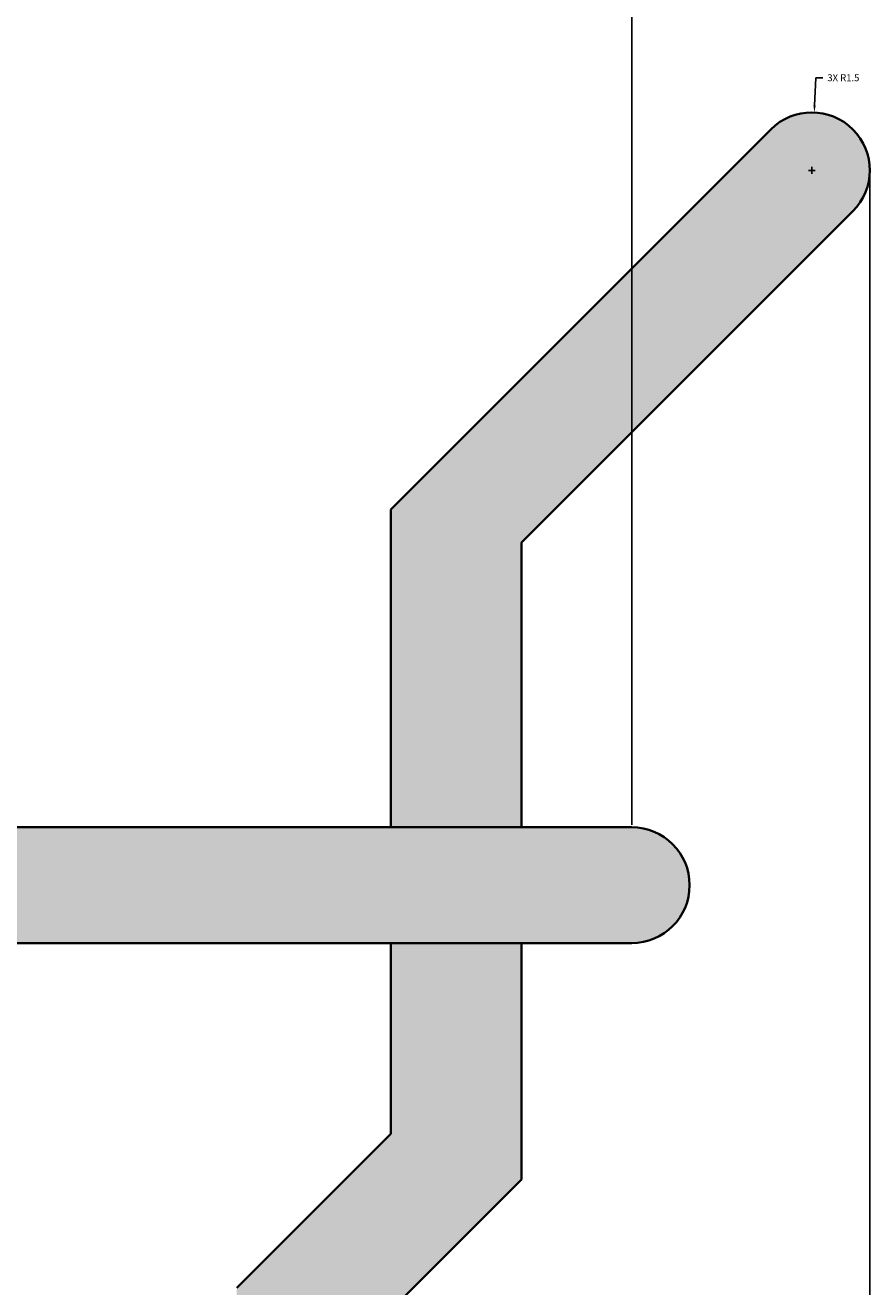
# Model space of a CAD drawing. Units: millimetres. Extents: x -11 to 280, y -4 to 208.
# Tile 37 of 55: x 244 to 266, y 23 to 55. Entities that reach past the tile are written whole.
import ezdxf

# ---------------------------------------------------------------- set-up
doc = ezdxf.new("R2010")
doc.units = ezdxf.units.MM
for name, color, linetype, lineweight in [('M-DIMS', 2, 'Continuous', 18), ('M-HYDR-CYL', 7, 'Continuous', 35), ('M-HYDR-CYL-PATT', 252, 'Continuous', 13)]:
    doc.layers.add(name, color=color, linetype=linetype, lineweight=lineweight)
doc.styles.get("Standard").update_dxf_attribs({"font": 'arial.ttf'})
doc.dimstyles.get("Standard").update_dxf_attribs({"dimtxt": 0.18, "dimasz": 0.18, "dimexe": 0.18, "dimexo": 0.0625, "dimgap": 0.09, "dimtad": 0, "dimtih": 1, "dimtoh": 1, "dimdec": 4, "dimzin": 0, "dimdsep": 46, "dimtxsty": 'Standard', "dimcen": 0.09, "dimadec": 0, "dimazin": 0, "dimtfac": 1, "dimtdec": 4, "dimtofl": 0, "dimtmove": 0, "dimatfit": 3, "dimfxl": 1, "dimtolj": 1, "dimtzin": 0, "dimarcsym": 0})

# ---------------------------------------------------------------- blocks, each defined once
blk = doc.blocks.new('*D4')
at = {"layer": 'Defpoints', "color": 0, "transparency": 16777216}
for p in [(4.763, 84.426), (266.035, 51.733), (266.035, -3.415)]:
    blk.add_point(p, dxfattribs=at)
at = {"layer": 'M-DIMS', "color": 0, "lineweight": -2, "transparency": 16777216}
for p, q in [((4.763, 84.364), (4.763, -3.595)), ((266.035, 51.67), (266.035, -3.595)), ((4.943, -3.415), (134.934, -3.415)), ((265.855, -3.415), (135.864, -3.415))]:
    blk.add_line(p, q, dxfattribs=at)
at = {"layer": 'M-DIMS', "color": 0, "transparency": 16777216}
for points in [[(4.943, -3.385), (4.943, -3.445), (4.763, -3.415)], [(265.855, -3.385), (265.855, -3.445), (266.035, -3.415)]]:
    blk.add_solid(points, dxfattribs=at)
at = {"layer": 'M-DIMS', "color": 0, "transparency": 16777216, "insert": (135.399, -3.415), "char_height": 0.18, "attachment_point": 5}
blk.add_mtext('\\A1;261.27', dxfattribs=at)
blk = doc.blocks.new('*D5')
at = {"layer": 'Defpoints', "color": 0, "transparency": 16777216}
for p in [(24.759, 192.645), (-10.087, 11.435), (261.686, 11.435)]:
    blk.add_point(p, dxfattribs=at)
at = {"layer": 'M-DIMS', "color": 0, "lineweight": -2, "transparency": 16777216}
for p, q in [((24.696, 192.645), (-10.267, 192.645)), ((-10.087, 192.465), (-10.087, 102.222)), ((-10.087, 11.615), (-10.087, 101.858)), ((261.624, 11.435), (-10.267, 11.435))]:
    blk.add_line(p, q, dxfattribs=at)
at = {"layer": 'M-DIMS', "color": 0, "transparency": 16777216}
for points in [[(-10.117, 192.465), (-10.057, 192.465), (-10.087, 192.645)], [(-10.117, 11.615), (-10.057, 11.615), (-10.087, 11.435)]]:
    blk.add_solid(points, dxfattribs=at)
at = {"layer": 'M-DIMS', "color": 0, "transparency": 16777216, "insert": (-10.087, 102.04), "char_height": 0.18, "attachment_point": 5}
blk.add_mtext('\\A1;181.2', dxfattribs=at)
blk = doc.blocks.new('*D22')
at = {"layer": 'Defpoints', "color": 0, "transparency": 16777216}
for p in [(259.871, 207.495), (231.68, 34.723), (259.871, 34.723)]:
    blk.add_point(p, dxfattribs=at)
at = {"layer": 'M-DIMS', "color": 0, "lineweight": -2, "transparency": 16777216}
for p, q in [((231.68, 34.785), (231.68, 207.675)), ((231.86, 207.495), (245.38, 207.495)), ((259.691, 207.495), (246.171, 207.495)), ((259.871, 34.785), (259.871, 207.675))]:
    blk.add_line(p, q, dxfattribs=at)
at = {"layer": 'M-DIMS', "color": 0, "transparency": 16777216}
for points in [[(231.86, 207.525), (231.86, 207.465), (231.68, 207.495)], [(259.691, 207.525), (259.691, 207.465), (259.871, 207.495)]]:
    blk.add_solid(points, dxfattribs=at)
at = {"layer": 'M-DIMS', "color": 0, "transparency": 16777216, "insert": (245.776, 207.495), "char_height": 0.18, "attachment_point": 5}
blk.add_mtext('\\A1;28.19', dxfattribs=at)
blk = doc.blocks.new('*D35')
at = {"layer": 'Defpoints', "color": 0, "transparency": 16777216}
for p in [(264.599, 53.235), (264.535, 51.736)]:
    blk.add_point(p, dxfattribs=at)
at = {"layer": 'M-DIMS', "color": 0, "lineweight": -2, "transparency": 16777216}
for p, q in [((264.638, 54.134), (264.607, 53.414)), ((264.818, 54.134), (264.638, 54.134)), ((264.445, 51.736), (264.625, 51.736)), ((264.535, 51.646), (264.535, 51.826))]:
    blk.add_line(p, q, dxfattribs=at)
at = {"layer": 'M-DIMS', "color": 0, "transparency": 16777216}
blk.add_solid([(264.577, 53.416), (264.637, 53.413), (264.599, 53.235)], dxfattribs=at)
at = {"layer": 'M-DIMS', "color": 0, "transparency": 16777216, "insert": (265.352, 54.134), "char_height": 0.18, "attachment_point": 5}
blk.add_mtext('\\A1;3X R1.5', dxfattribs=at)

msp = doc.modelspace()

# ---------------------------------------------------------------- hatches: boundary and pattern name
at = {"layer": 'M-HYDR-CYL-PATT'}
h = msp.add_hatch(color=256, dxfattribs=at)
h.set_gradient(color1=(128, 128, 128), color2=(99, 100, 102), tint=1)
h.paths.add_polyline_path([(163.0955, 41.5991), (160.6935, 41.5991), (160.6935, 24.846), (163.0955, 24.846)])
h.paths.add_polyline_path([(259.871, 34.7226), (163.0955, 34.7226), (163.0955, 31.7226), (259.871, 31.7226, 1)])
h.paths.add_polyline_path([(257.0171, 42.0966), (265.5958, 50.6754, 1), (263.4745, 52.7967), (253.6316, 42.9537), (253.6316, 34.7226), (257.0171, 34.7226)])
h.paths.add_polyline_path([(257.0171, 25.6028), (257.0171, 31.7226), (253.6316, 31.7226), (253.6316, 26.785), (249.6456, 22.7991), (249.6456, 13.7204, 1), (252.6456, 13.7204), (252.6456, 21.2313)])
h.paths.add_polyline_path([(265.4334, 20.9382), (261.6863, 20.9382), (261.6863, 11.4346), (265.4334, 11.4346)])
h.paths.add_polyline_path([(261.6863, 17.1598), (252.6456, 17.1598), (252.6456, 15.9126), (261.6863, 15.9126)])

# ---------------------------------------------------------------- linework, layer by layer
at = {"layer": 'M-HYDR-CYL'}
for p, q in [((253.6316, 42.9537), (263.4745, 52.7967)), ((265.5958, 50.6754), (257.0171, 42.0966)), ((253.6316, 34.7226), (253.6316, 42.9537)), ((257.0171, 42.0966), (257.0171, 34.7226)), ((259.871, 34.7226), (163.0955, 34.7226)), ((259.871, 31.7226), (163.0955, 31.7226)), ((253.6316, 26.785), (253.6316, 31.7226)), ((257.0171, 31.7226), (257.0171, 25.6028)), ((249.6456, 22.7991), (253.6316, 26.785)), ((257.0171, 25.6028), (252.6456, 21.2313))]:
    msp.add_line(p, q, dxfattribs=at)
for centre, start, end in [((264.5351, 51.736), 315, 135), ((259.871, 33.2226), 270, 90)]:
    msp.add_arc(centre, 1.5, start, end, dxfattribs=at)

# ---------------------------------------------------------------- dimensions: what is measured, and where the dimension line sits
at = {"layer": 'M-DIMS'}
for base, p1, p2, picture, middle in [((259.871, 207.495), (231.6803, 34.7226), (259.871, 34.7226), '*D22', (245.7757, 207.495)), ((266.0352, -3.4154), (4.7635, 84.4261), (266.0352, 51.7328), '*D4', (135.3993, -3.4154))]:
    dim = msp.add_linear_dim(base=base, p1=p1, p2=p2, dimstyle='Standard', override={"dimdec": 2, "dimlfac": 1, "dimrnd": 0, "dimzin": 0, "dimdsep": 46, "dimlunit": 2}, dxfattribs=at)
    dim.commit()
    dim.dimension.update_dxf_attribs({"geometry": picture, "text_midpoint": middle})
dim = msp.add_linear_dim(base=(-10.0865, 11.4346), p1=(24.7588, 192.645), p2=(261.6863, 11.4346), angle=90, dimstyle='Standard', override={"dimdec": 1, "dimlfac": 1, "dimrnd": 0, "dimzin": 0, "dimdsep": 46, "dimlunit": 2}, dxfattribs=at)
dim.commit()
dim.dimension.update_dxf_attribs({"geometry": '*D5', "text_midpoint": (-10.0865, 102.0398)})
dim = msp.add_radius_dim(center=(264.5351, 51.736), mpoint=(264.5993, 53.2346), text='3X <>', dimstyle='Standard', override={"dimdec": 1, "dimlfac": 1, "dimrnd": 0, "dimzin": 0, "dimdsep": 46, "dimlunit": 2}, dxfattribs=at)
dim.commit()
dim.dimension.update_dxf_attribs({"geometry": '*D35', "text_midpoint": (265.3518, 54.1338), "dimtype": 164})

doc.saveas('drawing.dxf')
